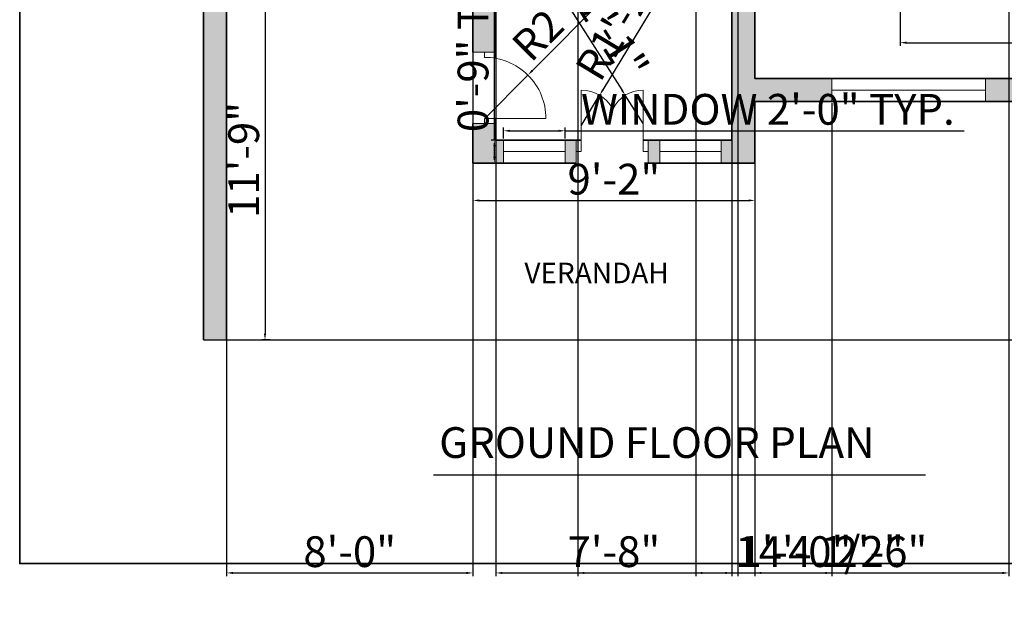
# Model space of a CAD drawing. Units: inches. Extents: x 995 to 1625, y 1005 to 1825.
# Tile 1 of 5: x 995 to 1379, y 1005 to 1232. Entities that reach past the tile are written whole.
import ezdxf

# ---------------------------------------------------------------- set-up
doc = ezdxf.new("R2010")
doc.units = ezdxf.units.IN
doc.linetypes.add('HIDDEN2', pattern=[4.7625, 3.175, -1.5875])
for name, color, linetype, lineweight in [('A-ANNO-DIMS', 2, 'Continuous', 18), ('A-ANNO-TEXT', 7, 'Continuous', 25), ('A-ANNO-TTLB', 7, 'Continuous', 35), ('A-AREA-IDEN', 7, 'Continuous', 18), ('A-DOOR', 4, 'Continuous', 18), ('A-FLOR-OVHD', 253, 'HIDDEN2', 18), ('A-GLAZ', 3, 'Continuous', 18), ('A-WALL', 7, 'Continuous', 35), ('C-PROP', 7, 'Continuous', 25)]:
    doc.layers.add(name, color=color, linetype=linetype, lineweight=lineweight)
doc.layers.add('A-WALL-PATT', color=251, linetype='Continuous', lineweight=13, true_color=0x636466)
doc.styles.get("Standard").update_dxf_attribs({"font": 'arial.ttf'})
doc.dimstyles.new('ISO-25', dxfattribs={"dimtxt": 12, "dimasz": 2.5, "dimexe": 1.25, "dimexo": 0.625, "dimtad": 1, "dimdec": 0, "dimlunit": 3, "dimtxsty": 'Standard', "dimcen": 2.5, "dimadec": 0, "dimazin": 0, "dimtfac": 1, "dimtdec": 0, "dimtmove": 0, "dimatfit": 3, "dimfxl": 1, "dimarcsym": 0})

# ---------------------------------------------------------------- blocks, each defined once
blk = doc.blocks.new('*D1')
at = {"layer": 'A-ANNO-DIMS', "color": 0, "lineweight": -2, "transparency": 16777216}
for p, q in [((1092.78, 1247.93), (1089.58, 1247.93)), ((1090.83, 1245.43), (1090.83, 1109.93)), ((1092.78, 1107.43), (1089.58, 1107.43))]:
    blk.add_line(p, q, dxfattribs=at)
at = {"layer": 'A-ANNO-DIMS', "color": 0, "transparency": 16777216}
for points in [[(1090.41, 1245.43), (1091.25, 1245.43), (1090.83, 1247.93)], [(1090.41, 1109.93), (1091.25, 1109.93), (1090.83, 1107.43)]]:
    blk.add_solid(points, dxfattribs=at)
at = {"layer": 'Defpoints', "color": 0, "transparency": 16777216}
for p in [(1093.41, 1247.93), (1090.83, 1107.43), (1093.41, 1107.43)]:
    blk.add_point(p, dxfattribs=at)
at = {"layer": 'A-ANNO-DIMS', "color": 0, "transparency": 16777216, "insert": (1084.08, 1177.68), "char_height": 12, "attachment_point": 5, "rotation": 90}
blk.add_mtext('11\'-9"', dxfattribs=at)
blk = doc.blocks.new('*D2')
at = {"layer": 'A-ANNO-DIMS', "color": 0, "lineweight": -2, "transparency": 16777216}
for p, q in [((1171.87, 1175.8), (1171.87, 1160.61)), ((1281.87, 1175.8), (1281.87, 1160.61)), ((1174.37, 1161.86), (1279.37, 1161.86))]:
    blk.add_line(p, q, dxfattribs=at)
at = {"layer": 'A-ANNO-DIMS', "color": 0, "transparency": 16777216}
for points in [[(1174.37, 1162.27), (1174.37, 1161.44), (1171.87, 1161.86)], [(1279.37, 1162.27), (1279.37, 1161.44), (1281.87, 1161.86)]]:
    blk.add_solid(points, dxfattribs=at)
at = {"layer": 'Defpoints', "color": 0, "transparency": 16777216}
for p in [(1171.87, 1176.43), (1281.87, 1176.43), (1281.87, 1161.86)]:
    blk.add_point(p, dxfattribs=at)
at = {"layer": 'A-ANNO-DIMS', "color": 0, "transparency": 16777216, "insert": (1226.87, 1168.61), "char_height": 12, "attachment_point": 5}
blk.add_mtext('9\'-2"', dxfattribs=at)
blk = doc.blocks.new('WIN-24IN')
for p, q in [((0, 0), (0, -9)), ((24, -4.5), (24, 0)), ((24, 0), (24, -9)), ((0, -9), (0, -4.5)), ((0, -4.5), (24, -4.5))]:
    blk.add_line(p, q)
blk = doc.blocks.new('WIN-60IN')
for p, q in [((0, 0), (9, 0)), ((9, 0), (4.5, 0)), ((4.5, 0), (4.5, -60)), ((4.5, -60), (0, -60)), ((0, -60), (9, -60))]:
    blk.add_line(p, q)
blk = doc.blocks.new('*D12')
at = {"layer": 'A-ANNO-DIMS', "color": 0, "lineweight": -2, "transparency": 16777216}
for p, q in [((1183.85, 1186.05), (1183.85, 1190.28)), ((1207.85, 1186.05), (1207.85, 1190.28)), ((1186.35, 1189.03), (1205.35, 1189.03)), ((1207.85, 1189.03), (1363.45, 1189.03))]:
    blk.add_line(p, q, dxfattribs=at)
at = {"layer": 'A-ANNO-DIMS', "color": 0, "transparency": 16777216}
for points in [[(1186.35, 1189.44), (1186.35, 1188.61), (1183.85, 1189.03)], [(1205.35, 1189.44), (1205.35, 1188.61), (1207.85, 1189.03)]]:
    blk.add_solid(points, dxfattribs=at)
at = {"layer": 'Defpoints', "color": 0, "transparency": 16777216}
for p in [(1207.85, 1189.03), (1183.85, 1185.43), (1207.85, 1185.43)]:
    blk.add_point(p, dxfattribs=at)
at = {"layer": 'A-ANNO-DIMS', "color": 0, "transparency": 16777216, "insert": (1286.9, 1195.86), "char_height": 12, "attachment_point": 5}
blk.add_mtext('WINDOW 2\'-0" TYP.', dxfattribs=at)
blk = doc.blocks.new('*D13')
at = {"layer": 'A-ANNO-DIMS', "color": 0, "lineweight": -2, "transparency": 16777216}
for p, q in [((1180.25, 1185.43), (1180.25, 1262.32)), ((1183.23, 1185.43), (1179, 1185.43)), ((1180.25, 1178.93), (1180.25, 1182.93)), ((1183.23, 1176.43), (1179, 1176.43))]:
    blk.add_line(p, q, dxfattribs=at)
at = {"layer": 'A-ANNO-DIMS', "color": 0, "transparency": 16777216}
for points in [[(1179.84, 1182.93), (1180.67, 1182.93), (1180.25, 1185.43)], [(1179.84, 1178.93), (1180.67, 1178.93), (1180.25, 1176.43)]]:
    blk.add_solid(points, dxfattribs=at)
at = {"layer": 'Defpoints', "color": 0, "transparency": 16777216}
for p in [(1180.25, 1185.43), (1183.85, 1185.43), (1183.85, 1176.43)]:
    blk.add_point(p, dxfattribs=at)
at = {"layer": 'A-ANNO-DIMS', "color": 0, "transparency": 16777216, "insert": (1173.5, 1225.13), "char_height": 12, "attachment_point": 5, "rotation": 90}
blk.add_mtext('0\'-9" TYP.', dxfattribs=at)
blk = doc.blocks.new('*D18')
at = {"layer": 'A-ANNO-DIMS', "color": 0, "lineweight": -2, "transparency": 16777216}
for p, q in [((1338.5, 1237.34), (1338.5, 1222.16)), ((1435.5, 1237.34), (1435.5, 1222.16)), ((1341, 1223.41), (1433, 1223.41)), ((1435.5, 1223.41), (1624.52, 1223.41))]:
    blk.add_line(p, q, dxfattribs=at)
at = {"layer": 'A-ANNO-DIMS', "color": 0, "transparency": 16777216}
for points in [[(1341, 1223.83), (1341, 1223), (1338.5, 1223.41)], [(1433, 1223.83), (1433, 1223), (1435.5, 1223.41)]]:
    blk.add_solid(points, dxfattribs=at)
at = {"layer": 'Defpoints', "color": 0, "transparency": 16777216}
for p in [(1338.5, 1237.96), (1435.5, 1237.96), (1435.5, 1223.41)]:
    blk.add_point(p, dxfattribs=at)
at = {"layer": 'A-ANNO-DIMS', "color": 0, "transparency": 16777216, "insert": (1531.26, 1230.25), "char_height": 12, "attachment_point": 5}
blk.add_mtext('DOUBLE BED 8\'-1" TYP.', dxfattribs=at)
blk = doc.blocks.new('*D24')
at = {"layer": 'A-ANNO-DIMS', "color": 0, "lineweight": -2, "transparency": 16777216}
for p, q in [((1075.87, 1247.3), (1075.87, 1015.27)), ((1171.87, 1247.3), (1171.87, 1015.27)), ((1078.37, 1016.52), (1169.37, 1016.52))]:
    blk.add_line(p, q, dxfattribs=at)
at = {"layer": 'A-ANNO-DIMS', "color": 0, "transparency": 16777216}
for points in [[(1078.37, 1016.93), (1078.37, 1016.1), (1075.87, 1016.52)], [(1169.37, 1016.93), (1169.37, 1016.1), (1171.87, 1016.52)]]:
    blk.add_solid(points, dxfattribs=at)
at = {"layer": 'Defpoints', "color": 0, "transparency": 16777216}
for p in [(1075.87, 1247.93), (1171.87, 1247.93), (1171.87, 1016.52)]:
    blk.add_point(p, dxfattribs=at)
at = {"layer": 'A-ANNO-DIMS', "color": 0, "transparency": 16777216, "insert": (1123.87, 1023.27), "char_height": 12, "attachment_point": 5}
blk.add_mtext('8\'-0"', dxfattribs=at)
blk = doc.blocks.new('*D30')
at = {"layer": 'A-ANNO-DIMS', "color": 0, "lineweight": -2, "transparency": 16777216}
for p, q in [((1212.87, 1517.8), (1212.87, 1015.27)), ((1380.87, 1517.8), (1380.87, 1015.27)), ((1215.37, 1016.52), (1378.37, 1016.52))]:
    blk.add_line(p, q, dxfattribs=at)
at = {"layer": 'A-ANNO-DIMS', "color": 0, "transparency": 16777216}
for points in [[(1215.37, 1016.93), (1215.37, 1016.1), (1212.87, 1016.52)], [(1378.37, 1016.93), (1378.37, 1016.1), (1380.87, 1016.52)]]:
    blk.add_solid(points, dxfattribs=at)
at = {"layer": 'Defpoints', "color": 0, "transparency": 16777216}
for p in [(1212.87, 1518.43), (1380.87, 1518.43), (1380.87, 1016.52)]:
    blk.add_point(p, dxfattribs=at)
at = {"layer": 'A-ANNO-DIMS', "color": 0, "transparency": 16777216, "insert": (1296.87, 1023.27), "char_height": 12, "attachment_point": 5}
blk.add_mtext('14\'-0"', dxfattribs=at)
blk = doc.blocks.new('*D32')
at = {"layer": 'A-ANNO-DIMS', "color": 0, "lineweight": -2, "transparency": 16777216}
for p, q in [((1180.87, 1340.8), (1180.87, 1015.27)), ((1272.87, 1340.8), (1272.87, 1015.27)), ((1183.37, 1016.52), (1270.37, 1016.52))]:
    blk.add_line(p, q, dxfattribs=at)
at = {"layer": 'A-ANNO-DIMS', "color": 0, "transparency": 16777216}
for points in [[(1183.37, 1016.93), (1183.37, 1016.1), (1180.87, 1016.52)], [(1270.37, 1016.93), (1270.37, 1016.1), (1272.87, 1016.52)]]:
    blk.add_solid(points, dxfattribs=at)
at = {"layer": 'Defpoints', "color": 0, "transparency": 16777216}
for p in [(1180.87, 1341.43), (1272.87, 1341.43), (1272.87, 1016.52)]:
    blk.add_point(p, dxfattribs=at)
at = {"layer": 'A-ANNO-DIMS', "color": 0, "transparency": 16777216, "insert": (1226.87, 1023.27), "char_height": 12, "attachment_point": 5}
blk.add_mtext('7\'-8"', dxfattribs=at)
blk = doc.blocks.new('*D37')
at = {"layer": 'A-ANNO-DIMS', "color": 0, "lineweight": -2, "transparency": 16777216}
for p, q in [((1258.87, 1658.8), (1258.87, 1015.27)), ((1275.16, 1658.8), (1275.16, 1015.27)), ((1261.37, 1016.52), (1272.66, 1016.52)), ((1275.16, 1016.52), (1337.64, 1016.52))]:
    blk.add_line(p, q, dxfattribs=at)
at = {"layer": 'A-ANNO-DIMS', "color": 0, "transparency": 16777216}
for points in [[(1261.37, 1016.93), (1261.37, 1016.1), (1258.87, 1016.52)], [(1272.66, 1016.93), (1272.66, 1016.1), (1275.16, 1016.52)]]:
    blk.add_solid(points, dxfattribs=at)
at = {"layer": 'Defpoints', "color": 0, "transparency": 16777216}
for p in [(1258.87, 1659.43), (1275.16, 1659.43), (1275.16, 1016.52)]:
    blk.add_point(p, dxfattribs=at)
at = {"layer": 'A-ANNO-DIMS', "color": 0, "transparency": 16777216, "insert": (1307.65, 1023.35), "char_height": 12, "attachment_point": 5}
blk.add_mtext('1\'-4 1/2"', dxfattribs=at)
blk = doc.blocks.new('*D42')
at = {"layer": 'A-ANNO-DIMS', "color": 0, "lineweight": -2, "transparency": 16777216}
for p, q in [((1281.87, 1199.8), (1281.87, 1015.27)), ((1311.82, 1199.8), (1311.82, 1015.27)), ((1284.37, 1016.52), (1309.32, 1016.52)), ((1311.82, 1016.52), (1347.68, 1016.52))]:
    blk.add_line(p, q, dxfattribs=at)
at = {"layer": 'A-ANNO-DIMS', "color": 0, "transparency": 16777216}
for points in [[(1284.37, 1016.93), (1284.37, 1016.1), (1281.87, 1016.52)], [(1309.32, 1016.93), (1309.32, 1016.1), (1311.82, 1016.52)]]:
    blk.add_solid(points, dxfattribs=at)
at = {"layer": 'Defpoints', "color": 0, "transparency": 16777216}
for p in [(1281.87, 1200.43), (1311.82, 1200.43), (1311.82, 1016.52)]:
    blk.add_point(p, dxfattribs=at)
at = {"layer": 'A-ANNO-DIMS', "color": 0, "transparency": 16777216, "insert": (1331, 1023.27), "char_height": 12, "attachment_point": 5}
blk.add_mtext('2\'-6"', dxfattribs=at)
blk = doc.blocks.new('*D50')
at = {"layer": 'A-ANNO-DIMS', "color": 0, "lineweight": -2, "transparency": 16777216}
for p, q in [((1228.3, 1245.97), (1195.09, 1212.53)), ((1176.53, 1193.84), (1193.33, 1210.75))]:
    blk.add_line(p, q, dxfattribs=at)
at = {"layer": 'A-ANNO-DIMS', "color": 0, "transparency": 16777216}
blk.add_solid([(1194.79, 1212.82), (1195.38, 1212.23), (1193.33, 1210.75)], dxfattribs=at)
at = {"layer": 'Defpoints', "color": 0, "transparency": 16777216}
for p in [(1193.33, 1210.75), (1176.53, 1193.84)]:
    blk.add_point(p, dxfattribs=at)
at = {"layer": 'A-ANNO-DIMS', "color": 0, "transparency": 16777216, "insert": (1207.79, 1234.89), "char_height": 12, "attachment_point": 5, "rotation": 45.1957}
blk.add_mtext('R2\'-0"', dxfattribs=at)
blk = doc.blocks.new('*D54')
at = {"layer": 'A-ANNO-DIMS', "color": 0, "lineweight": -2, "transparency": 16777216}
for p, q in [((1246.99, 1245.39), (1222.61, 1205.06)), ((1214.11, 1191), (1221.31, 1202.92))]:
    blk.add_line(p, q, dxfattribs=at)
at = {"layer": 'A-ANNO-DIMS', "color": 0, "transparency": 16777216}
blk.add_solid([(1222.25, 1205.27), (1222.96, 1204.84), (1221.31, 1202.92)], dxfattribs=at)
at = {"layer": 'Defpoints', "color": 0, "transparency": 16777216}
for p in [(1221.31, 1202.92), (1214.11, 1191)]:
    blk.add_point(p, dxfattribs=at)
at = {"layer": 'A-ANNO-DIMS', "color": 0, "transparency": 16777216, "insert": (1229.75, 1229.74), "char_height": 12, "attachment_point": 5, "rotation": 58.8445}
blk.add_mtext('R1\'-2"', dxfattribs=at)
blk = doc.blocks.new('*D55')
at = {"layer": 'A-ANNO-DIMS', "color": 0, "lineweight": -2, "transparency": 16777216}
for p, q in [((1204.75, 1244.87), (1229.92, 1205.02)), ((1238.24, 1191.86), (1231.26, 1202.91))]:
    blk.add_line(p, q, dxfattribs=at)
at = {"layer": 'A-ANNO-DIMS', "color": 0, "transparency": 16777216}
blk.add_solid([(1230.28, 1205.24), (1229.57, 1204.8), (1231.26, 1202.91)], dxfattribs=at)
at = {"layer": 'Defpoints', "color": 0, "transparency": 16777216}
for p in [(1231.26, 1202.91), (1238.24, 1191.86)]:
    blk.add_point(p, dxfattribs=at)
at = {"layer": 'A-ANNO-DIMS', "color": 0, "transparency": 16777216, "insert": (1222.29, 1229.55), "char_height": 12, "attachment_point": 5, "rotation": 302.2824}
blk.add_mtext('R1\'-1"', dxfattribs=at)

msp = doc.modelspace()

# ---------------------------------------------------------------- hatches: boundary and pattern name
at = {"layer": 'A-WALL-PATT'}
h = msp.add_hatch(color=256, dxfattribs=at)
h.dxf.hatch_style = 1
h.paths.add_polyline_path([(1446.87, 1737.43), (1066.87, 1737.43), (1066.87, 1718.28), (1075.87, 1718.28), (1075.87, 1728.43), (1171.87, 1728.43), (1171.87, 1668.43), (1165.05, 1668.43), (1165.05, 1659.43), (1219.13, 1659.43), (1219.13, 1663.93), (1219.13, 1668.43), (1180.87, 1668.43), (1180.87, 1691.88), (1180.87, 1728.43), (1249.87, 1728.43), (1258.87, 1728.43), (1332.87, 1728.43), (1332.87, 1668.43), (1311.16, 1668.43), (1311.16, 1659.43), (1346.35, 1659.43), (1346.35, 1663.93), (1346.35, 1668.43), (1341.87, 1668.43), (1341.87, 1728.43), (1437.87, 1728.43), (1437.87, 1715.56), (1446.87, 1715.56)])
h.paths.add_polyline_path([(1135.58, 1663.93), (1135.58, 1668.43), (1075.87, 1668.43), (1075.87, 1694.28), (1066.87, 1694.28), (1066.87, 1619.54), (1075.87, 1619.54), (1075.87, 1659.43), (1135.58, 1659.43)])
h.paths.add_polyline_path([(1258.87, 1659.43), (1275.16, 1659.43), (1275.16, 1663.93), (1275.16, 1668.43), (1258.87, 1668.43), (1249.87, 1668.43), (1243.74, 1668.43), (1243.74, 1659.43), (1249.87, 1659.43), (1249.87, 1527.43), (1247.75, 1527.43), (1247.75, 1518.43), (1261.81, 1518.43), (1261.81, 1527.43), (1258.87, 1527.43)])
h.paths.add_polyline_path([(1446.87, 1691.56), (1437.87, 1691.56), (1437.87, 1668.43), (1372.6, 1668.43), (1372.6, 1659.43), (1437.87, 1659.43), (1437.87, 1627.58), (1446.87, 1627.58)])
h.paths.add_polyline_path([(1446.87, 1567.58), (1437.87, 1567.58), (1437.87, 1527.43), (1291.03, 1527.43), (1291.03, 1518.43), (1380.87, 1518.43), (1380.87, 1508.92), (1389.87, 1508.92), (1389.87, 1518.43), (1437.87, 1518.43), (1437.87, 1501.62), (1446.87, 1501.62)])
h.paths.add_polyline_path([(1446.87, 1477.62), (1437.87, 1477.62), (1437.87, 1429.75), (1446.87, 1429.75)])
h.paths.add_polyline_path([(1389.87, 1441.43), (1437.87, 1441.43), (1437.87, 1450.43), (1389.87, 1450.43), (1389.87, 1481.88), (1385.37, 1481.88), (1380.87, 1481.88), (1380.87, 1385.88), (1389.87, 1385.88)])
h.paths.add_polyline_path([(1446.87, 1405.75), (1437.87, 1405.75), (1437.87, 1350.43), (1427.33, 1350.43), (1389.87, 1350.43), (1389.87, 1359.9), (1380.87, 1359.9), (1380.87, 1350.43), (1324.85, 1350.43), (1324.85, 1341.43), (1437.87, 1341.43), (1437.87, 1303.84), (1446.87, 1303.84)])
h.paths.add_polyline_path([(1311.82, 1209.43), (1281.87, 1209.43), (1281.87, 1341.43), (1291.29, 1341.43), (1291.29, 1345.93), (1291.29, 1350.43), (1244.83, 1350.43), (1244.83, 1341.43), (1272.87, 1341.43), (1272.87, 1185.43), (1268.73, 1185.43), (1268.73, 1176.43), (1272.87, 1176.43), (1281.87, 1176.43), (1281.87, 1200.43), (1311.82, 1200.43), (1311.82, 1204.93)])
h.paths.add_polyline_path([(1446.87, 1243.84), (1437.87, 1243.84), (1437.87, 1209.43), (1371.82, 1209.43), (1371.82, 1200.43), (1437.87, 1200.43), (1437.87, 1107.43), (1446.87, 1107.43)])
h.paths.add_polyline_path([(1212.11, 1185.43), (1207.85, 1185.43), (1207.85, 1176.43), (1212.11, 1176.43)], flags=17)
h.paths.add_polyline_path([(1244.73, 1185.43), (1240.24, 1185.43), (1240.24, 1176.43), (1244.73, 1176.43), (1244.73, 1180.93)])
h.paths.add_polyline_path([(1183.85, 1180.93), (1183.85, 1185.43), (1180.87, 1185.43), (1180.87, 1191.84), (1171.87, 1191.84), (1171.87, 1176.43), (1180.87, 1176.43), (1183.85, 1176.43)], flags=17)
h.paths.add_polyline_path([(1180.87, 1341.43), (1198.57, 1341.43), (1198.57, 1350.43), (1180.87, 1350.43), (1180.87, 1354.13), (1176.37, 1354.13), (1171.87, 1354.13), (1171.87, 1341.43), (1171.87, 1219.68), (1180.87, 1219.68)], flags=17)
h.paths.add_polyline_path([(1075.87, 1391.93), (1171.87, 1391.93), (1171.87, 1389.24), (1180.87, 1389.24), (1180.87, 1391.93), (1212.87, 1391.93), (1212.87, 1431.83), (1203.87, 1431.83), (1203.87, 1400.93), (1075.87, 1400.93), (1075.87, 1446.29), (1066.87, 1446.29), (1066.87, 1107.43), (1075.87, 1107.43)])
h.paths.add_polyline_path([(1218.33, 1527.43), (1075.87, 1527.43), (1075.87, 1559.54), (1066.87, 1559.54), (1066.87, 1482.29), (1075.87, 1482.29), (1075.87, 1518.43), (1203.87, 1518.43), (1203.87, 1493.65), (1212.87, 1493.65), (1212.87, 1518.43), (1218.33, 1518.43), (1218.33, 1522.93)])
h.paths.add_polyline_path([(1297.68, 1457.37), (1297.68, 1425.03), (1310.04, 1425.03), (1310.04, 1457.37)], flags=9)
h.paths.add_polyline_path([(1154.86, 1054.62), (1346.22, 1054.62), (1346.22, 1079.35), (1154.86, 1079.35)], flags=9)
h.paths.add_polyline_path([(1237.85, 1265.85), (1262.06, 1265.85), (1262.06, 1288.24), (1237.85, 1288.24)], flags=9)
h.paths.add_polyline_path([(1331.39, 1305.41), (1378, 1305.41), (1378, 1327.8), (1331.39, 1327.8)], flags=25)
h.paths.add_polyline_path([(1395.38, 1378.18), (1431.86, 1378.18), (1431.86, 1400.57), (1395.38, 1400.57)], flags=25)
h.paths.add_polyline_path([(1406.34, 1460.18), (1434.48, 1460.18), (1434.48, 1472.55), (1406.34, 1472.55)], flags=25)
h.paths.add_polyline_path([(1134.66, 1454.9), (1180.38, 1454.9), (1180.38, 1477.29), (1134.66, 1477.29)], flags=9)
h.paths.add_polyline_path([(1109.63, 1626.32), (1156.23, 1626.32), (1156.23, 1648.71), (1109.63, 1648.71)], flags=9)
h.paths.add_polyline_path([(1275.64, 1623.22), (1322.25, 1623.22), (1322.25, 1645.61), (1275.64, 1645.61)], flags=9)
h.paths.add_polyline_path([(1347.7, 1693.6), (1384.09, 1693.6), (1384.09, 1715.99), (1347.7, 1715.99)], flags=25)
h.paths.add_polyline_path([(1254.21, 1701.46), (1308.94, 1701.46), (1308.94, 1723.85), (1254.21, 1723.85)], flags=25)
h.paths.add_polyline_path([(1107.35, 1692.25), (1143.74, 1692.25), (1143.74, 1714.64), (1107.35, 1714.64)], flags=25)

# ---------------------------------------------------------------- linework, layer by layer
at = {"layer": 'A-ANNO-TEXT'}
msp.add_line((1156.59, 1054.77), (1348.3, 1054.77), dxfattribs=at)
at = {"layer": 'A-ANNO-TTLB'}
msp.add_lwpolyline([(995.18, 1825.14), (1553.05, 1825.14), (1553.05, 1020.2), (995.18, 1020.2)], close=True, dxfattribs=at)
at = {"layer": 'A-DOOR'}
for p, q in [((1171.87, 1219.68), (1180.87, 1219.68)), ((1180.87, 1219.68), (1176.37, 1219.68)), ((1176.37, 1219.68), (1176.37, 1217.68)), ((1214.11, 1180.93), (1214.11, 1204.93)), ((1238.24, 1180.93), (1238.24, 1204.93)), ((1180.87, 1191.84), (1171.87, 1191.84)), ((1171.87, 1191.84), (1176.37, 1191.84)), ((1176.37, 1191.84), (1176.37, 1193.84)), ((1176.37, 1193.84), (1200.37, 1193.84)), ((1212.11, 1185.43), (1212.11, 1176.43)), ((1240.24, 1185.43), (1240.24, 1176.43)), ((1212.11, 1180.93), (1214.11, 1180.93)), ((1240.24, 1180.93), (1238.24, 1180.93))]:
    msp.add_line(p, q, dxfattribs=at)
for centre, radius, start, end in [((1176.53, 1193.84), 23.84, 0, 90.3924), ((1214.11, 1191), 13.92, 27.6873, 90), ((1238.24, 1191.86), 13.06, 90, 154.566)]:
    msp.add_arc(centre, radius, start, end, dxfattribs=at)
at = {"layer": 'A-FLOR-OVHD'}
for p, q in [((1171.87, 1176.43), (1171.87, 1107.43)), ((1281.87, 1176.43), (1281.87, 1107.43))]:
    msp.add_line(p, q, dxfattribs=at)
at = {"layer": 'A-WALL'}
for p, q in [((1066.87, 1737.43), (1066.87, 1107.43)), ((1066.87, 1737.43), (1066.87, 1107.43)), ((1066.87, 1737.43), (1066.87, 1107.43)), ((1075.87, 1391.93), (1075.87, 1107.43)), ((1171.87, 1341.43), (1171.87, 1219.68)), ((1180.87, 1341.43), (1180.87, 1217.28)), ((1272.87, 1341.43), (1272.87, 1185.43)), ((1281.87, 1341.43), (1281.87, 1209.43)), ((1281.87, 1209.43), (1437.87, 1209.43)), ((1281.87, 1200.43), (1437.87, 1200.43)), ((1281.87, 1200.43), (1281.87, 1176.43)), ((1171.87, 1191.84), (1171.87, 1176.43)), ((1180.87, 1193.84), (1180.87, 1185.43)), ((1180.87, 1185.43), (1214.11, 1185.43)), ((1238.24, 1185.43), (1272.87, 1185.43)), ((1180.87, 1176.43), (1171.87, 1176.43)), ((1180.87, 1176.43), (1212.11, 1176.43)), ((1240.24, 1176.43), (1272.87, 1176.43)), ((1272.87, 1176.43), (1281.87, 1176.43))]:
    msp.add_line(p, q, dxfattribs=at)
at = {"layer": 'C-PROP'}
msp.add_line((1066.87, 1107.43), (1446.87, 1107.43), dxfattribs=at)

# ---------------------------------------------------------------- block references
at = {"layer": 'A-GLAZ', "extrusion": (0, 0, -1), "zscale": -1, "rotation": 270}
msp.add_blockref('WIN-60IN', (-1311.82, 1209.43), dxfattribs=at)
at = {"layer": 'A-GLAZ'}
for p in [(1183.85, 1185.43), (1244.73, 1185.43)]:
    msp.add_blockref('WIN-24IN', p, dxfattribs=at)

# ---------------------------------------------------------------- texts
at = {"layer": 'A-ANNO-TEXT', "insert": (1158.75, 1073.39), "char_height": 12, "attachment_point": 1}
msp.add_mtext_dynamic_manual_height_columns('GROUND FLOOR PLAN', width=350.4205, gutter_width=12.5, heights=[0], dxfattribs=at)
at = {"layer": 'A-AREA-IDEN', "insert": (1191.97, 1137.58), "char_height": 8, "attachment_point": 1}
msp.add_mtext_dynamic_manual_height_columns('VERANDAH', width=79.8556, gutter_width=12.5, heights=[0], dxfattribs=at)

# ---------------------------------------------------------------- dimensions: what is measured, and where the dimension line sits
at = {"layer": 'A-ANNO-DIMS'}
for base, p1, p2, override, picture, middle in [((1275.16, 1016.52), (1258.87, 1659.43), (1275.16, 1659.43), {"dimdec": 1, "dimlfac": 1, "dimrnd": 0, "dimzin": 1, "dimdsep": 46, "dimlunit": 4, "dimfrac": 2}, '*D37', (1307.65, 1023.35)), ((1380.87, 1016.52), (1212.87, 1518.43), (1380.87, 1518.43), {"dimdec": 1, "dimlfac": 1, "dimrnd": 0, "dimzin": 1, "dimdsep": 46, "dimlunit": 4, "dimfrac": 2}, '*D30', (1296.87, 1023.27)), ((1272.87, 1016.52), (1180.87, 1341.43), (1272.87, 1341.43), {"dimdec": 1, "dimlfac": 1, "dimrnd": 0, "dimzin": 1, "dimdsep": 46, "dimlunit": 4, "dimfrac": 2}, '*D32', (1226.87, 1023.27)), ((1171.87, 1016.52), (1075.87, 1247.93), (1171.87, 1247.93), {"dimdec": 1, "dimlfac": 1, "dimrnd": 0, "dimzin": 1, "dimdsep": 46, "dimlunit": 4, "dimfrac": 2}, '*D24', (1123.87, 1023.27)), ((1311.8248, 1016.5161), (1281.8661, 1200.4271), (1311.8248, 1200.4271), {"dimdec": 1, "dimlfac": 1, "dimrnd": 0, "dimzin": 1, "dimdsep": 46, "dimlunit": 4, "dimfrac": 2}, '*D42', (1331.0017, 1023.268)), ((1281.87, 1161.86), (1171.87, 1176.43), (1281.87, 1176.43), {"dimclrd": 0, "dimclre": 0, "dimclrt": 0}, '*D2', (1226.87, 1168.61))]:
    dim = msp.add_linear_dim(base=base, p1=p1, p2=p2, dimstyle='ISO-25', override=override, dxfattribs=at)
    dim.commit()
    dim.dimension.update_dxf_attribs({"geometry": picture, "text_midpoint": middle})
for base, p1, p2, text, picture, middle in [((1435.5, 1223.41), (1338.5, 1237.96), (1435.5, 1237.96), 'DOUBLE BED <> TYP.', '*D18', (1531.26, 1230.25)), ((1207.85, 1189.03), (1183.85, 1185.43), (1207.85, 1185.43), 'WINDOW <> TYP.', '*D12', (1286.9, 1195.86))]:
    dim = msp.add_linear_dim(base=base, p1=p1, p2=p2, text=text, dimstyle='ISO-25', override={"dimdec": 1, "dimlfac": 1, "dimrnd": 0, "dimzin": 1, "dimdsep": 46, "dimlunit": 4, "dimfrac": 2}, dxfattribs=at)
    dim.commit()
    dim.dimension.update_dxf_attribs({"geometry": picture, "text_midpoint": middle})
dim = msp.add_linear_dim(base=(1180.25, 1185.43), p1=(1183.85, 1176.43), p2=(1183.85, 1185.43), angle=90, text='<> TYP.', dimstyle='ISO-25', override={"dimdec": 1, "dimlfac": 1, "dimrnd": 0, "dimzin": 1, "dimdsep": 46, "dimlunit": 4, "dimfrac": 2}, dxfattribs=at)
dim.commit()
dim.dimension.update_dxf_attribs({"geometry": '*D13', "text_midpoint": (1173.5, 1225.13)})
for center, mpoint, picture, middle in [((1176.53, 1193.84), (1193.33, 1210.75), '*D50', (1207.79, 1234.89)), ((1238.24, 1191.86), (1231.26, 1202.91), '*D55', (1222.29, 1229.55)), ((1214.11, 1191), (1221.31, 1202.92), '*D54', (1229.75, 1229.74))]:
    dim = msp.add_radius_dim(center=center, mpoint=mpoint, dimstyle='ISO-25', override={"dimdec": 1, "dimlfac": 1, "dimrnd": 0, "dimzin": 1, "dimdsep": 46, "dimlunit": 4, "dimfrac": 2}, dxfattribs=at)
    dim.commit()
    dim.dimension.update_dxf_attribs({"geometry": picture, "text_midpoint": middle})
dim = msp.add_linear_dim(base=(1090.8307, 1107.4271), p1=(1093.4057, 1247.928), p2=(1093.4057, 1107.4271), angle=90, dimstyle='ISO-25', override={"dimclrd": 0, "dimclre": 0, "dimclrt": 0}, dxfattribs=at)
dim.commit()
dim.dimension.update_dxf_attribs({"geometry": '*D1', "text_midpoint": (1090.8307, 1177.6775), "dimtype": 160})

doc.saveas('drawing.dxf')
